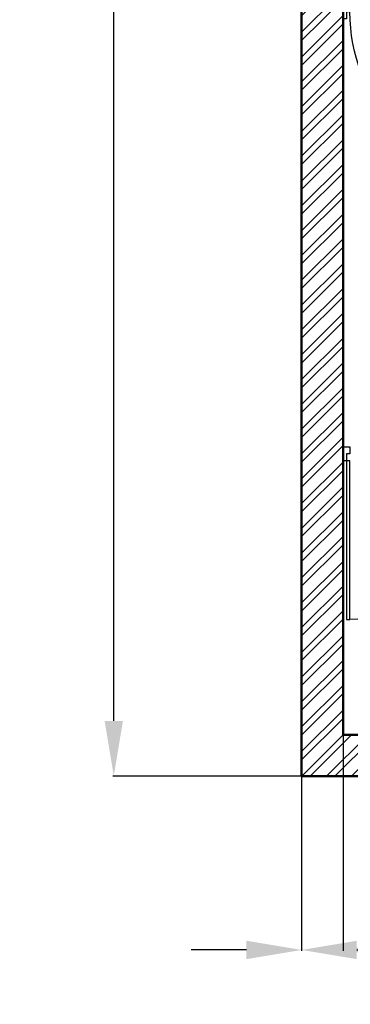
# Model space of a CAD drawing. Units: inches. Extents: x -90 to 536, y -553 to 299.
# Tile 1 of 27: x -23 to 49, y -553 to -339. Entities that reach past the tile are written whole.
import ezdxf

# ---------------------------------------------------------------- set-up
doc = ezdxf.new("R2010")
doc.units = ezdxf.units.IN
for name, color, linetype, lineweight in [('A-ANNO-DIMS', 2, 'Continuous', 18), ('A-DOOR', 4, 'Continuous', 25), ('A-WALL-PATT', 252, 'Continuous', 13), ('Outer Wall', 1, 'Continuous', 50)]:
    doc.layers.add(name, color=color, linetype=linetype, lineweight=lineweight)
doc.styles.get("Standard").update_dxf_attribs({"font": 'arial.ttf'})
doc.dimstyles.get("Standard").update_dxf_attribs({"dimtxt": 18, "dimasz": 12, "dimexe": 0.18, "dimexo": 0.0625, "dimgap": 0.09, "dimtad": 0, "dimtih": 1, "dimtoh": 1, "dimdec": 0, "dimzin": 0, "dimdsep": 46, "dimlunit": 3, "dimtxsty": 'Standard', "dimcen": 0.09, "dimadec": 0, "dimazin": 0, "dimtfac": 1, "dimtdec": 0, "dimtofl": 0, "dimtmove": 0, "dimatfit": 3, "dimfxl": 1, "dimtolj": 1, "dimtzin": 0, "dimarcsym": 0})

# ---------------------------------------------------------------- blocks, each defined once
blk = doc.blocks.new('DOOR-36-A')
for points in [[(35.25, 37.5), (35.25, 3), (34.5, 3), (34.5, 37.5)], [(0, 0), (1.5, 0), (1.5, 1.5), (0.75, 1.5), (0.75, 3), (0, 3)], [(36, 0), (34.5, 0), (34.5, 1.5), (35.25, 1.5), (35.25, 3), (36, 3)]]:
    blk.add_lwpolyline(points, close=True)
blk.add_arc((37.64, 1.5), 36.14, 94.9791, 180)
blk = doc.blocks.new('DOOR-36-B')
for points in [[(37.5, 36), (37.5, 34.5), (36, 34.5), (36, 35.25), (34.5, 35.25), (34.5, 36)], [(0, 0.75), (0, 1.5), (34.5, 1.5), (34.5, 0.75)], [(37.5, 0), (37.5, 1.5), (36, 1.5), (36, 0.75), (34.5, 0.75), (34.5, 0)]]:
    blk.add_lwpolyline(points, close=True)
blk.add_arc((33.76, 1.5), 33.76, 88.7408, 180)
blk = doc.blocks.new('*D54')
at = {"layer": 'A-ANNO-DIMS', "color": 0, "lineweight": -2, "transparency": 16777216}
for p, q in [((113.07, 249.45), (-2.85, 249.45)), ((-2.67, 237.45), (-2.67, -117.77)), ((-2.67, -491.55), (-2.67, -136.34)), ((38.07, -503.55), (-2.85, -503.55))]:
    blk.add_line(p, q, dxfattribs=at)
at = {"layer": 'A-ANNO-DIMS', "color": 0, "transparency": 16777216}
for points in [[(-4.67, 237.45), (-0.67, 237.45), (-2.67, 249.45)], [(-4.67, -491.55), (-0.67, -491.55), (-2.67, -503.55)]]:
    blk.add_solid(points, dxfattribs=at)
at = {"layer": 'Defpoints', "color": 0, "transparency": 16777216}
for p in [(-2.67, 249.45), (113.13, 249.45), (38.13, -503.55)]:
    blk.add_point(p, dxfattribs=at)
at = {"layer": 'A-ANNO-DIMS', "color": 0, "transparency": 16777216, "insert": (-2.67, -127.05), "char_height": 18, "attachment_point": 5}
blk.add_mtext('\\A1;753', dxfattribs=at)
blk = doc.blocks.new('*D57')
at = {"layer": 'A-ANNO-DIMS', "color": 0, "lineweight": -2, "transparency": 16777216}
for p, q in [((47.13, -494.62), (47.13, -541.49)), ((38.13, -503.62), (38.13, -541.49)), ((26.13, -541.31), (14.13, -541.31)), ((59.13, -541.31), (71.13, -541.31))]:
    blk.add_line(p, q, dxfattribs=at)
at = {"layer": 'A-ANNO-DIMS', "color": 0, "transparency": 16777216}
for points in [[(26.13, -539.31), (26.13, -543.31), (38.13, -541.31)], [(59.13, -539.31), (59.13, -543.31), (47.13, -541.31)]]:
    blk.add_solid(points, dxfattribs=at)
at = {"layer": 'Defpoints', "color": 0, "transparency": 16777216}
for p in [(47.13, -494.55), (38.13, -503.55), (47.13, -541.31)]:
    blk.add_point(p, dxfattribs=at)
at = {"layer": 'A-ANNO-DIMS', "color": 0, "transparency": 16777216, "insert": (77.14, -541.31), "char_height": 18, "attachment_point": 5}
blk.add_mtext('\\A1;9', dxfattribs=at)
blk = doc.blocks.new('*D67')
at = {"layer": 'A-ANNO-DIMS', "color": 0, "lineweight": -2, "transparency": 16777216}
for p, q in [((261.13, -437.62), (261.13, -541.49)), ((38.13, -503.62), (38.13, -541.49)), ((50.13, -541.31), (129.5, -541.31)), ((249.13, -541.31), (169.76, -541.31))]:
    blk.add_line(p, q, dxfattribs=at)
at = {"layer": 'A-ANNO-DIMS', "color": 0, "transparency": 16777216}
for points in [[(50.13, -539.31), (50.13, -543.31), (38.13, -541.31)], [(249.13, -539.31), (249.13, -543.31), (261.13, -541.31)]]:
    blk.add_solid(points, dxfattribs=at)
at = {"layer": 'Defpoints', "color": 0, "transparency": 16777216}
for p in [(261.13, -437.55), (38.13, -503.55), (261.13, -541.31)]:
    blk.add_point(p, dxfattribs=at)
at = {"layer": 'A-ANNO-DIMS', "color": 0, "transparency": 16777216, "insert": (149.63, -541.31), "char_height": 18, "attachment_point": 5}
blk.add_mtext('\\A1;223', dxfattribs=at)

msp = doc.modelspace()

# ---------------------------------------------------------------- hatches: boundary and pattern name
at = {"layer": 'A-WALL-PATT'}
h = msp.add_hatch(dxfattribs=at)
h.set_pattern_fill('ANSI32', color=256, scale=0.4)
h.set_pattern_definition([(45, (-88.8105, -603.6155), (-2.694077, 2.694077), []), (45, (-87.0145, -603.6155), (-2.694077, 2.694077), [])])
h.paths.add_polyline_path([(285.1317, 246.4462), (131.1317, 246.4462), (131.1317, 237.4462), (285.1317, 237.4462)])
h.paths.add_polyline_path([(122.1317, 237.4462), (113.1317, 237.4462), (113.1317, 152.4462), (122.1317, 152.4462), (122.1317, 166.4704)])
h.paths.add_polyline_path([(303.1317, 237.4462), (294.1317, 237.4462), (294.1317, 152.4462), (303.1317, 152.4462)])
h.paths.add_polyline_path([(47.1317, 91.9277), (38.1317, 91.9277), (38.1317, -6.5538), (77.1317, -6.5538), (77.1317, 2.4462), (70.5655, 2.4462), (47.1317, 2.4462)])
h.paths.add_polyline_path([(83.052, -61.5538), (47.1317, -61.5538), (47.1317, -24.5538), (38.1317, -24.5538), (38.1317, -70.5538), (74.052, -70.5538), (74.052, -223.5538), (38.1317, -223.5538), (38.1317, -503.5538), (92.1317, -503.5538), (92.1317, -437.5538), (191.1317, -437.5538), (191.1317, -428.5538), (83.1317, -428.5538), (83.1317, -494.5538), (47.1317, -494.5538), (47.1317, -232.5538), (83.052, -232.5538), (83.052, -70.5538)])
h.paths.add_polyline_path([(407.1317, -63.5538), (381.1317, -63.5538), (381.1317, 91.9277), (372.1317, 91.9277), (372.1317, 32.8805), (372.1317, -63.5538), (306.5745, -63.5538), (237.1317, -63.5538), (237.1317, -38.5538), (233.1317, -38.5538), (233.1317, -71.5538), (398.1317, -71.5538), (398.1317, -152.5538), (233.1317, -152.5538), (233.1317, -161.5538), (398.1317, -161.5538), (398.1317, -368.5538), (233.1317, -368.5538), (233.1317, -377.5538), (407.1317, -377.5538), (407.1317, -161.5538)])
h.paths.add_polyline_path([(261.1317, -422.5538), (252.1317, -422.5538), (252.1317, -428.5538), (233.1317, -428.5538), (233.1317, -437.5538), (261.1317, -437.5538)])
h.paths.add_polyline_path([(191.1317, -368.5538), (180.1317, -368.5538), (180.1317, -335.5538), (131.5919, -335.5538), (131.5919, -344.5538), (171.1317, -344.5538), (171.1317, -392.5538), (180.1317, -392.5538), (180.1317, -377.5538), (191.1317, -377.5538)], flags=17)
h.paths.add_polyline_path([(180.1317, -223.5538), (152.1317, -223.5538), (152.1317, -227.5538), (176.1317, -227.5538), (176.1317, -335.5538), (180.1317, -335.5538)], flags=17)
h.paths.add_polyline_path([(131.5919, -335.5538), (83.1317, -335.5538), (83.1317, -339.5538), (83.1317, -392.5538), (87.1317, -392.5538), (87.1317, -339.5538), (131.5919, -339.5538)], flags=17)
h.paths.add_polyline_path([(197.1317, 2.4462), (77.1317, 2.4462), (77.1317, -1.5538), (113.1317, -1.5538), (113.1317, -71.5538), (181.1317, -71.5538), (181.1317, -67.5538), (117.1317, -67.5538), (117.1317, -1.5538), (177.1317, -1.5538), (177.1317, -37.5538), (181.1317, -37.5538), (181.1317, -1.5538), (197.1317, -1.5538)])
h.paths.add_polyline_path([(173.1317, 138.4462), (122.1317, 138.4462), (122.1317, 134.4462), (173.1317, 134.4462)])
h.paths.add_polyline_path([(213.1317, 237.4462), (209.1317, 237.4462), (209.1317, 134.4462), (233.1317, 134.4462), (233.1317, 68.8889), (233.1317, -2.5538), (237.1317, -2.5538), (237.1317, 134.4462), (258.1317, 134.4462), (258.1317, 138.4462), (213.1317, 138.4462)])

# ---------------------------------------------------------------- linework, layer by layer
at = {"layer": 'Outer Wall'}
for p, q in [((38.1317, -223.5538), (38.1317, -503.5538)), ((47.1317, -232.5538), (47.1317, -494.5538)), ((83.1317, -494.5538), (47.1317, -494.5538)), ((92.1317, -503.5538), (38.1317, -503.5538))]:
    msp.add_line(p, q, dxfattribs=at)

# ---------------------------------------------------------------- block references
at = {"layer": 'A-DOOR', "extrusion": (0, 0, -1), "zscale": -1}
for name, p, rotation in [('DOOR-36-A', (-47.1317, -336.0538), 180), ('DOOR-36-B', (-47.1317, -469.529), 89.99999999999979)]:
    msp.add_blockref(name, p, dxfattribs=dict(at, rotation=rotation))

# ---------------------------------------------------------------- dimensions: what is measured, and where the dimension line sits
at = {"layer": 'A-ANNO-DIMS'}
dim = msp.add_linear_dim(base=(-2.6677, 249.4462), p1=(38.1317, -503.5538), p2=(113.1317, 249.4462), angle=90, dimstyle='Standard', override={"dimdec": 0, "dimlfac": 1, "dimrnd": 0, "dimzin": 0, "dimdsep": 46, "dimlunit": 2}, dxfattribs=at)
dim.commit()
dim.dimension.update_dxf_attribs({"geometry": '*D54', "text_midpoint": (-2.6677, -127.0538)})
for base, p2, picture, middle in [((261.1317, -541.3088), (261.1317, -437.5538), '*D67', (149.6317, -541.3088)), ((47.1317, -541.3088), (47.1317, -494.5538), '*D57', (77.1399, -541.3088))]:
    dim = msp.add_linear_dim(base=base, p1=(38.1317, -503.5538), p2=p2, dimstyle='Standard', override={"dimdec": 0, "dimlfac": 1, "dimrnd": 0, "dimzin": 0, "dimdsep": 46, "dimlunit": 2}, dxfattribs=at)
    dim.commit()
    dim.dimension.update_dxf_attribs({"geometry": picture, "text_midpoint": middle})

doc.saveas('drawing.dxf')
